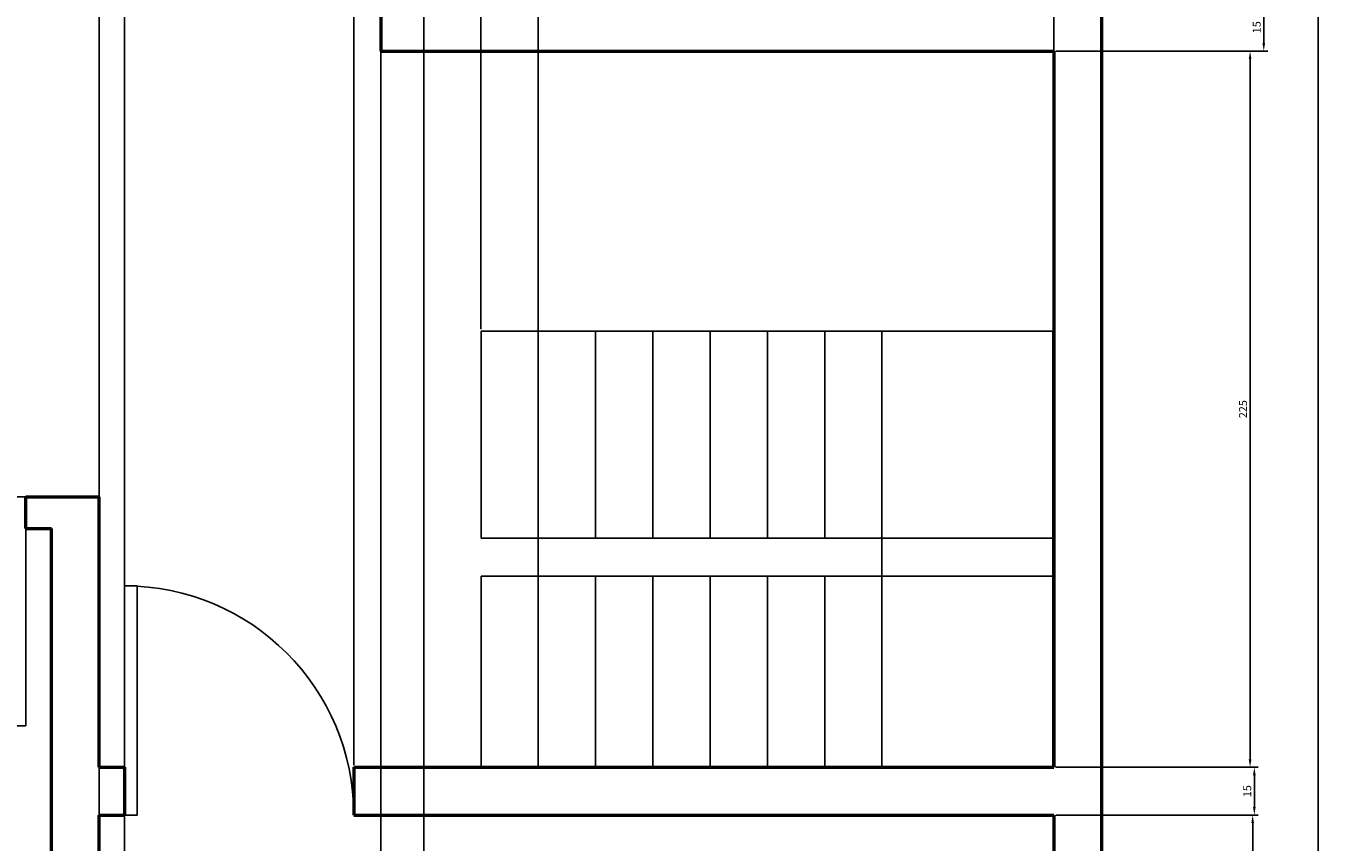
# Model space of a CAD drawing. Units: inches. Extents: x 604 to 3492, y -123 to 1737.
# Tile 15 of 20: x 1912 to 2319, y 579 to 836. Entities that reach past the tile are written whole.
import ezdxf

# ---------------------------------------------------------------- set-up
doc = ezdxf.new("R2010")
doc.units = ezdxf.units.IN
for name, color, linetype, lineweight in [('A-ANNO-DIMS', 2, 'Continuous', 18), ('A-DOOR', 3, 'Continuous', 25), ('A-FLOR-STRS', 7, 'Continuous', 25), ('A-WALL', 7, 'Continuous', 50)]:
    doc.layers.add(name, color=color, linetype=linetype, lineweight=lineweight)
doc.styles.get("Standard").update_dxf_attribs({"font": 'arial.ttf'})
doc.dimstyles.new('ISO-25', dxfattribs={"dimtxt": 2.5, "dimasz": 2.5, "dimexe": 1.25, "dimexo": 0.625, "dimtad": 1, "dimtxsty": 'Standard', "dimcen": 2.5, "dimadec": 0, "dimazin": 0, "dimtfac": 1, "dimtmove": 0, "dimatfit": 3, "dimfxl": 1, "dimarcsym": 0})

# ---------------------------------------------------------------- blocks, each defined once
blk = doc.blocks.new('*D47')
at = {"layer": 'A-ANNO-DIMS', "color": 0, "lineweight": -2, "transparency": 16777216}
for p, q in [((2235.2, 842.7), (2301.8, 842.7)), ((2300.55, 840.2), (2300.55, 830.2)), ((2235.2, 827.7), (2301.8, 827.7))]:
    blk.add_line(p, q, dxfattribs=at)
at = {"layer": 'A-ANNO-DIMS', "color": 0, "transparency": 16777216}
for points in [[(2300.13, 840.2), (2300.96, 840.2), (2300.55, 842.7)], [(2300.13, 830.2), (2300.96, 830.2), (2300.55, 827.7)]]:
    blk.add_solid(points, dxfattribs=at)
at = {"layer": 'Defpoints', "color": 0, "transparency": 16777216}
for p in [(2234.57, 842.7), (2234.57, 827.7), (2300.55, 827.7)]:
    blk.add_point(p, dxfattribs=at)
at = {"layer": 'A-ANNO-DIMS', "color": 0, "transparency": 16777216, "insert": (2298.64, 835.2), "char_height": 2.5, "attachment_point": 5, "rotation": 90}
blk.add_mtext('15', dxfattribs=at)
blk = doc.blocks.new('*D48')
at = {"layer": 'A-ANNO-DIMS', "color": 0, "lineweight": -2, "transparency": 16777216}
for p, q in [((2235.2, 827.7), (2297.49, 827.7)), ((2296.24, 825.2), (2296.24, 605.2)), ((2235.2, 602.7), (2297.49, 602.7))]:
    blk.add_line(p, q, dxfattribs=at)
at = {"layer": 'A-ANNO-DIMS', "color": 0, "transparency": 16777216}
for points in [[(2295.82, 825.2), (2296.66, 825.2), (2296.24, 827.7)], [(2295.82, 605.2), (2296.66, 605.2), (2296.24, 602.7)]]:
    blk.add_solid(points, dxfattribs=at)
at = {"layer": 'Defpoints', "color": 0, "transparency": 16777216}
for p in [(2234.57, 827.7), (2234.57, 602.7), (2296.24, 602.7)]:
    blk.add_point(p, dxfattribs=at)
at = {"layer": 'A-ANNO-DIMS', "color": 0, "transparency": 16777216, "insert": (2294.34, 715.2), "char_height": 2.5, "attachment_point": 5, "rotation": 90}
blk.add_mtext('225', dxfattribs=at)
blk = doc.blocks.new('*D49')
at = {"layer": 'A-ANNO-DIMS', "color": 0, "lineweight": -2, "transparency": 16777216}
for p, q in [((2235.2, 602.7), (2298.83, 602.7)), ((2297.58, 600.2), (2297.58, 590.2)), ((2235.2, 587.7), (2298.83, 587.7))]:
    blk.add_line(p, q, dxfattribs=at)
at = {"layer": 'A-ANNO-DIMS', "color": 0, "transparency": 16777216}
for points in [[(2297.16, 600.2), (2298, 600.2), (2297.58, 602.7)], [(2297.16, 590.2), (2298, 590.2), (2297.58, 587.7)]]:
    blk.add_solid(points, dxfattribs=at)
at = {"layer": 'Defpoints', "color": 0, "transparency": 16777216}
for p in [(2234.57, 602.7), (2234.57, 587.7), (2297.58, 587.7)]:
    blk.add_point(p, dxfattribs=at)
at = {"layer": 'A-ANNO-DIMS', "color": 0, "transparency": 16777216, "insert": (2295.68, 595.2), "char_height": 2.5, "attachment_point": 5, "rotation": 90}
blk.add_mtext('15', dxfattribs=at)
blk = doc.blocks.new('*D50')
at = {"layer": 'A-ANNO-DIMS', "color": 0, "lineweight": -2, "transparency": 16777216}
for p, q in [((2235.2, 587.7), (2298.31, 587.7)), ((2297.06, 585.2), (2297.06, 470.2)), ((2235.2, 467.7), (2298.31, 467.7))]:
    blk.add_line(p, q, dxfattribs=at)
at = {"layer": 'A-ANNO-DIMS', "color": 0, "transparency": 16777216}
for points in [[(2296.64, 585.2), (2297.48, 585.2), (2297.06, 587.7)], [(2296.64, 470.2), (2297.48, 470.2), (2297.06, 467.7)]]:
    blk.add_solid(points, dxfattribs=at)
at = {"layer": 'Defpoints', "color": 0, "transparency": 16777216}
for p in [(2234.57, 587.7), (2234.57, 467.7), (2297.06, 467.7)]:
    blk.add_point(p, dxfattribs=at)
at = {"layer": 'A-ANNO-DIMS', "color": 0, "transparency": 16777216, "insert": (2295.16, 527.7), "char_height": 2.5, "attachment_point": 5, "rotation": 90}
blk.add_mtext('120', dxfattribs=at)
blk = doc.blocks.new('*D70')
at = {"layer": 'A-ANNO-DIMS', "color": 0, "lineweight": -2, "transparency": 16777216}
for p, q in [((2250.2, 1287.7), (2318.86, 1287.7)), ((2317.61, 455.2), (2317.61, 1285.2)), ((2250.2, 452.7), (2318.86, 452.7))]:
    blk.add_line(p, q, dxfattribs=at)
at = {"layer": 'A-ANNO-DIMS', "color": 0, "transparency": 16777216}
for points in [[(2317.2, 1285.2), (2318.03, 1285.2), (2317.61, 1287.7)], [(2317.2, 455.2), (2318.03, 455.2), (2317.61, 452.7)]]:
    blk.add_solid(points, dxfattribs=at)
at = {"layer": 'Defpoints', "color": 0, "transparency": 16777216}
for p in [(2249.57, 1287.7), (2317.61, 1287.7), (2249.57, 452.7)]:
    blk.add_point(p, dxfattribs=at)
at = {"layer": 'A-ANNO-DIMS', "color": 0, "transparency": 16777216, "insert": (2315.71, 870.2), "char_height": 2.5, "attachment_point": 5, "rotation": 90}
blk.add_mtext('835', dxfattribs=at)
blk = doc.blocks.new('DOOR-SWING-72')
for p, q in [((0, 72), (0, 0)), ((0, 0), (4, 0)), ((0, 0), (4, 0))]:
    blk.add_line(p, q)
blk.add_lwpolyline([(0, 72), (0, 0), (4, 0), (4, 72)], close=True)
blk.add_arc((0, 0), 72, 0, 90)
blk = doc.blocks.new('*D102')
at = {"layer": 'A-ANNO-DIMS', "color": 0, "lineweight": -2, "transparency": 16777216}
for p, q in [((1839.57, 972.08), (1839.57, 215.5)), ((2023.07, 972.08), (2023.07, 215.5)), ((1842.07, 216.75), (2020.57, 216.75))]:
    blk.add_line(p, q, dxfattribs=at)
at = {"layer": 'A-ANNO-DIMS', "color": 0, "transparency": 16777216}
for points in [[(1842.07, 217.17), (1842.07, 216.33), (1839.57, 216.75)], [(2020.57, 217.17), (2020.57, 216.33), (2023.07, 216.75)]]:
    blk.add_solid(points, dxfattribs=at)
at = {"layer": 'Defpoints', "color": 0, "transparency": 16777216}
for p in [(1839.57, 972.7), (2023.07, 972.7), (2023.07, 216.75)]:
    blk.add_point(p, dxfattribs=at)
at = {"layer": 'A-ANNO-DIMS', "color": 0, "transparency": 16777216, "insert": (1931.32, 218.65), "char_height": 2.5, "attachment_point": 5}
blk.add_mtext('183.5', dxfattribs=at)
blk = doc.blocks.new('*D104')
at = {"layer": 'A-ANNO-DIMS', "color": 0, "lineweight": -2, "transparency": 16777216}
for p, q in [((1934.57, 1272.08), (1934.57, 215.5)), ((2036.57, 1272.08), (2036.57, 215.5)), ((1937.07, 216.75), (2034.07, 216.75))]:
    blk.add_line(p, q, dxfattribs=at)
at = {"layer": 'A-ANNO-DIMS', "color": 0, "transparency": 16777216}
for points in [[(1937.07, 217.17), (1937.07, 216.33), (1934.57, 216.75)], [(2034.07, 217.17), (2034.07, 216.33), (2036.57, 216.75)]]:
    blk.add_solid(points, dxfattribs=at)
at = {"layer": 'Defpoints', "color": 0, "transparency": 16777216}
for p in [(1934.57, 1272.7), (2036.57, 1272.7), (2036.57, 216.75)]:
    blk.add_point(p, dxfattribs=at)
at = {"layer": 'A-ANNO-DIMS', "color": 0, "transparency": 16777216, "insert": (1985.57, 218.65), "char_height": 2.5, "attachment_point": 5}
blk.add_mtext('102', dxfattribs=at)
blk = doc.blocks.new('*D109')
at = {"layer": 'A-ANNO-DIMS', "color": 0, "lineweight": -2, "transparency": 16777216}
for p, q in [((2054.57, 740.33), (2054.57, 1359.9)), ((2057.07, 1358.65), (2232.07, 1358.65)), ((2234.57, 740.33), (2234.57, 1359.9))]:
    blk.add_line(p, q, dxfattribs=at)
at = {"layer": 'A-ANNO-DIMS', "color": 0, "transparency": 16777216}
for points in [[(2057.07, 1359.07), (2057.07, 1358.23), (2054.57, 1358.65)], [(2232.07, 1359.07), (2232.07, 1358.23), (2234.57, 1358.65)]]:
    blk.add_solid(points, dxfattribs=at)
at = {"layer": 'Defpoints', "color": 0, "transparency": 16777216}
for p in [(2234.57, 1358.65), (2054.57, 739.7), (2234.57, 739.7)]:
    blk.add_point(p, dxfattribs=at)
at = {"layer": 'A-ANNO-DIMS', "color": 0, "transparency": 16777216, "insert": (2144.57, 1360.55), "char_height": 2.5, "attachment_point": 5}
blk.add_mtext('180', dxfattribs=at)
blk = doc.blocks.new('*D112')
at = {"layer": 'A-ANNO-DIMS', "color": 0, "lineweight": -2, "transparency": 16777216}
for p, q in [((1934.57, 972.08), (1934.57, 215.5)), ((1942.57, 962.08), (1942.57, 215.5)), ((1940.07, 216.75), (1937.07, 216.75))]:
    blk.add_line(p, q, dxfattribs=at)
at = {"layer": 'A-ANNO-DIMS', "color": 0, "transparency": 16777216}
for points in [[(1937.07, 217.17), (1937.07, 216.33), (1934.57, 216.75)], [(1940.07, 217.17), (1940.07, 216.33), (1942.57, 216.75)]]:
    blk.add_solid(points, dxfattribs=at)
at = {"layer": 'Defpoints', "color": 0, "transparency": 16777216}
for p in [(1934.57, 972.7), (1942.57, 962.7), (1934.57, 216.75)]:
    blk.add_point(p, dxfattribs=at)
at = {"layer": 'A-ANNO-DIMS', "color": 0, "transparency": 16777216, "insert": (1938.57, 218.65), "char_height": 2.5, "attachment_point": 5}
blk.add_mtext('8', dxfattribs=at)
blk = doc.blocks.new('*D113')
at = {"layer": 'A-ANNO-DIMS', "color": 0, "lineweight": -2, "transparency": 16777216}
for p, q in [((2014.57, 603.33), (2014.57, 1359.9)), ((2017.07, 1358.65), (2070.07, 1358.65)), ((2072.57, 603.33), (2072.57, 1359.9))]:
    blk.add_line(p, q, dxfattribs=at)
at = {"layer": 'A-ANNO-DIMS', "color": 0, "transparency": 16777216}
for points in [[(2017.07, 1359.07), (2017.07, 1358.23), (2014.57, 1358.65)], [(2070.07, 1359.07), (2070.07, 1358.23), (2072.57, 1358.65)]]:
    blk.add_solid(points, dxfattribs=at)
at = {"layer": 'Defpoints', "color": 0, "transparency": 16777216}
for p in [(2072.57, 1358.65), (2014.57, 602.7), (2072.57, 602.7)]:
    blk.add_point(p, dxfattribs=at)
at = {"layer": 'A-ANNO-DIMS', "color": 0, "transparency": 16777216, "insert": (2043.57, 1360.55), "char_height": 2.5, "attachment_point": 5}
blk.add_mtext('58', dxfattribs=at)

msp = doc.modelspace()

# ---------------------------------------------------------------- linework, layer by layer
at = {"layer": 'A-FLOR-STRS'}
for p, q in [((2174.5743, 739.7004), (2054.5743, 739.7004)), ((2054.5743, 739.7004), (2054.5743, 674.7004)), ((2072.5743, 739.7004), (2072.5743, 674.7004)), ((2072.5743, 739.7004), (2072.5743, 674.7004)), ((2090.5743, 739.7004), (2090.5743, 674.7004)), ((2090.5743, 739.7004), (2090.5743, 674.7004)), ((2090.5743, 739.7004), (2090.5743, 674.7004)), ((2108.5743, 739.7004), (2108.5743, 674.7004)), ((2108.5743, 739.7004), (2108.5743, 674.7004)), ((2126.5743, 739.7004), (2126.5743, 674.7004)), ((2126.5743, 739.7004), (2126.5743, 674.7004)), ((2144.5743, 739.7004), (2144.5743, 674.7004)), ((2144.5743, 739.7004), (2144.5743, 674.7004)), ((2162.5743, 739.7004), (2162.5743, 674.7004)), ((2162.5743, 739.7004), (2162.5743, 674.7004)), ((2174.5743, 739.7004), (2234.5743, 739.7004)), ((2180.5743, 739.7004), (2180.5743, 674.7004)), ((2054.5743, 674.7004), (2180.5743, 674.7004)), ((2180.5743, 667.7004), (2180.5743, 674.7004)), ((2180.5743, 674.7004), (2234.5743, 674.7004)), ((2180.5743, 667.7004), (2180.5743, 602.7004)), ((2054.5743, 662.7004), (2180.5743, 662.7004)), ((2054.5743, 662.7004), (2054.5743, 602.7004)), ((2072.5743, 662.7004), (2072.5743, 602.7004)), ((2072.5743, 662.7004), (2072.5743, 602.7004)), ((2090.5743, 662.7004), (2090.5743, 602.7004)), ((2090.5743, 662.7004), (2090.5743, 602.7004)), ((2090.5743, 662.7004), (2090.5743, 602.7004)), ((2108.5743, 662.7004), (2108.5743, 602.7004)), ((2126.5743, 662.7004), (2126.5743, 602.7004)), ((2144.5743, 662.7004), (2144.5743, 602.7004)), ((2162.5743, 662.7004), (2162.5743, 602.7004)), ((2162.5743, 662.7004), (2162.5743, 602.7004)), ((2180.5743, 662.7004), (2234.5743, 662.7004))]:
    msp.add_line(p, q, dxfattribs=at)
at = {"layer": 'A-WALL'}
for p, q in [((2249.5743, 1287.7004), (2249.5743, 452.7004)), ((2023.0743, 842.7004), (2023.0743, 827.7004)), ((2023.0743, 827.7004), (2234.5743, 827.7004)), ((2023.0743, 827.7004), (2234.5743, 827.7004)), ((2234.5743, 827.7004), (2234.5743, 602.7004)), ((2234.5743, 602.7004), (2234.5743, 739.7004)), ((1911.5743, 677.7004), (1911.5743, 687.7004)), ((1911.5743, 687.7004), (1919.5743, 687.7004)), ((1919.5743, 687.7004), (1934.5743, 687.7004)), ((1934.5743, 602.7004), (1934.5743, 687.7004)), ((1911.5743, 677.7004), (1919.5743, 677.7004)), ((1919.5743, 302.7004), (1919.5743, 677.7004)), ((1934.5743, 602.7004), (1942.5743, 602.7004)), ((1942.5743, 602.7004), (1942.5743, 587.7004)), ((2014.5743, 602.7004), (2014.5743, 587.7004)), ((2014.5743, 602.7004), (2234.5743, 602.7004)), ((1934.5743, 587.7004), (1942.5743, 587.7004)), ((1934.5743, 467.7004), (1934.5743, 587.7004)), ((2014.5743, 587.7004), (2234.5743, 587.7004)), ((2234.5743, 587.7004), (2234.5743, 467.7004))]:
    msp.add_line(p, q, dxfattribs=at)

# ---------------------------------------------------------------- block references
at = {"layer": 'A-DOOR', "rotation": 180}
msp.add_blockref('DOOR-SWING-72', (1911.5743, 687.7004), dxfattribs=at)
at = {"layer": 'A-DOOR'}
msp.add_blockref('DOOR-SWING-72', (1942.5743, 587.7004), dxfattribs=at)

# ---------------------------------------------------------------- dimensions: what is measured, and where the dimension line sits
at = {"layer": 'A-ANNO-DIMS'}
for base, p1, p2, override, picture, middle in [((2072.5743, 1358.6504), (2014.5743, 602.7004), (2072.5743, 602.7004), {"dimdec": 0, "dimlfac": 1, "dimrnd": 0, "dimzin": 0, "dimdsep": 46, "dimlunit": 2}, '*D113', (2043.5743, 1360.5519)), ((2234.5743, 1358.6504), (2054.5743, 739.7004), (2234.5743, 739.7004), {"dimdec": 0, "dimlfac": 1, "dimrnd": 0, "dimzin": 0, "dimdsep": 46, "dimlunit": 2}, '*D109', (2144.5743, 1360.5519)), ((2036.5743, 216.7504), (1934.5743, 1272.7004), (2036.5743, 1272.7004), {"dimdec": 0, "dimlfac": 1, "dimrnd": 0, "dimzin": 0, "dimdsep": 46, "dimlunit": 2}, '*D104', (1985.5743, 218.6519)), ((2023.0743, 216.7504), (1839.5743, 972.7004), (2023.0743, 972.7004), {"dimdec": 1, "dimlfac": 1, "dimrnd": 0, "dimzin": 0, "dimdsep": 46, "dimlunit": 2}, '*D102', (1931.3243, 218.6527)), ((1934.5743, 216.7504), (1942.5743, 962.7004), (1934.5743, 972.7004), {"dimdec": 0, "dimlfac": 1, "dimrnd": 0, "dimzin": 0, "dimdsep": 46, "dimlunit": 2}, '*D112', (1938.5743, 218.6519))]:
    dim = msp.add_linear_dim(base=base, p1=p1, p2=p2, dimstyle='ISO-25', override=override, dxfattribs=at)
    dim.commit()
    dim.dimension.update_dxf_attribs({"geometry": picture, "text_midpoint": middle})
for p1, p2, distance, picture, middle in [((2249.5743, 452.7004), (2249.5743, 1287.7004), -68.0392, '*D70', (2315.7113, 870.2004)), ((2234.5743, 827.7004), (2234.5743, 602.7004), 61.6657, '*D48', (2294.3386, 715.2004))]:
    dim = msp.add_aligned_dim(p1=p1, p2=p2, distance=distance, dimstyle='ISO-25', override={"dimclrd": 0, "dimclre": 0, "dimclrt": 0}, dxfattribs=at)
    dim.commit()
    dim.dimension.update_dxf_attribs({"geometry": picture, "text_midpoint": middle})
for base, p1, p2, picture, middle in [((2300.5456, 827.7004), (2234.5743, 842.7004), (2234.5743, 827.7004), '*D47', (2298.6442, 835.2004)), ((2297.5793, 587.7004), (2234.5743, 602.7004), (2234.5743, 587.7004), '*D49', (2295.6779, 595.2004)), ((2297.0616, 467.7004), (2234.5743, 587.7004), (2234.5743, 467.7004), '*D50', (2295.1601, 527.7004))]:
    dim = msp.add_linear_dim(base=base, p1=p1, p2=p2, angle=90, dimstyle='ISO-25', override={"dimclrd": 0, "dimclre": 0, "dimclrt": 0}, dxfattribs=at)
    dim.commit()
    dim.dimension.update_dxf_attribs({"geometry": picture, "text_midpoint": middle})

doc.saveas('drawing.dxf')
